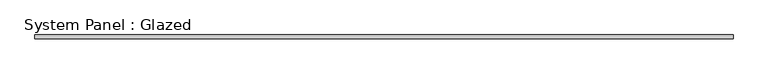
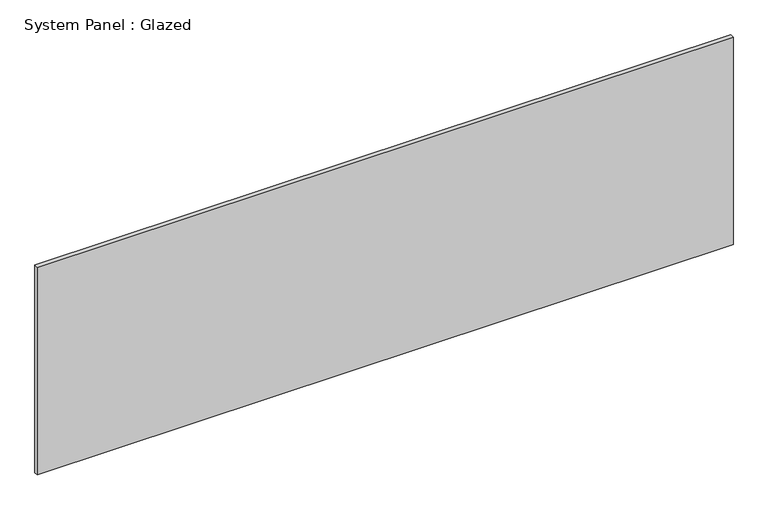
"""IFC4 building model written with IfcOpenShell, lengths in millimetres: plate geometry, System Panel : Glazed."""

from ifc_helpers import new_model, si_unit, origin, origin_with_axes, place, context, project, spatial, polyline, outline, extrude, source, transform, mapped, element, save


def system_panel_glazed_f6bd2989(model_context):
    return source(origin(), model_context, "Body", "SweptSolid", [
        extrude(outline(polyline([(2314.575, 19.05), (-2314.575, 19.05), (-2314.575, 44.45), (2314.575, 44.45), (2314.575, 19.05)])), origin_with_axes(), (0.0, 0.0, 1.0), 1460.5),
    ])


if __name__ == "__main__":
    model = new_model("IFC4")
    model_context = context("Model", 3, world=origin())
    ifc_project = project(units=[si_unit("LENGTHUNIT", "METRE", prefix="MILLI")], contexts=[model_context])
    site = spatial("IfcSite", under=ifc_project)
    building = spatial("IfcBuilding", under=site)
    placement = place(None, origin())
    system_panel_glazed_shape = system_panel_glazed_f6bd2989(model_context)
    element("IfcPlate", 1, ObjectType="System Panel : Glazed", at=placement, inside=building, context=model_context, shape_type="MappedRepresentation", body=[
        mapped(system_panel_glazed_shape, transform((0.0, 0.0, 0.0), x_axis=(1.0, 0.0, 0.0), y_axis=(0.0, 1.0, 0.0), z_axis=(0.0, 0.0, 1.0))),
    ])
    save(model, "model.ifc")

# Revit data of these elements
# Type "System Panel : Glazed"
#   Construction Type Id = "GSP4R"
#   Analytic Construction = "1/8 in Pilkington single glazing"
#   Visual Light Transmittance = 0.9
#   Solar Heat Gain Coefficient = 0.86
#   Heat Transfer Coefficient (U) = 1.18115 BTU/(h·ft²·°F)
# Element 1 (IfcPlate, "System Panel : Glazed")
#   Materials on its faces: "Glass"
# Materials
#   "Glass": class "Glass", colour RGB 0 128 192, transparency 0.75, Description = "Soda Lime Glass", Cost = 0
